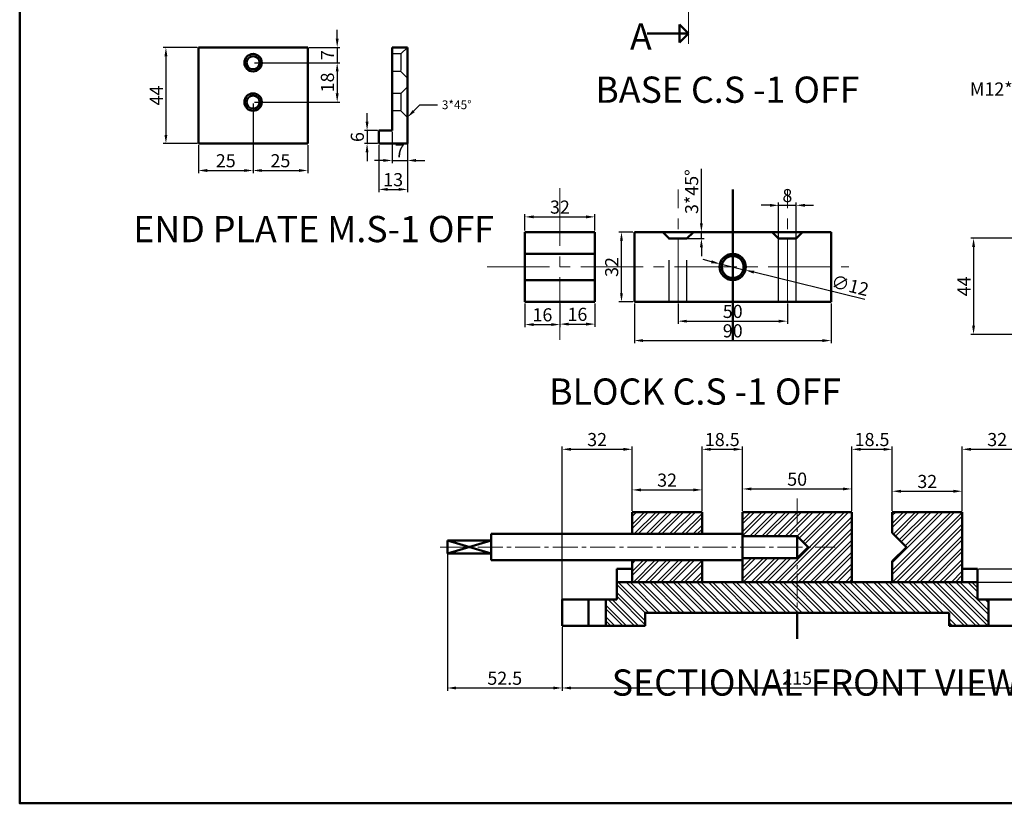
# Model space of a CAD drawing. Units: millimetres. Extents: x -1209 to -333, y 66 to 707.
# Tile 1 of 4: x -1209 to -759, y 66 to 424. Entities that reach past the tile are written whole.
import ezdxf
from ezdxf import colors
from ezdxf.entities.mleader import LeaderData, LeaderLine
from ezdxf.math import Vec2, Vec3

# ---------------------------------------------------------------- set-up
doc = ezdxf.new("R2010")
doc.units = ezdxf.units.MM
doc.header["$LTSCALE"] = 1.5
doc.linetypes.add('CENTER2', pattern=[28.575, 19.05, -3.175, 3.175, -3.175])
doc.linetypes.add('DASHED', pattern=[19.05, 12.7, -6.35])
for name, color, linetype, lineweight in [('M-CNTR', 1, 'CENTER2', 18), ('M-DIMS', 2, 'Continuous', 25), ('M-HATC', 8, 'Continuous', 18), ('M-HIDN', 4, 'DASHED', 25), ('M-OUTL', 7, 'Continuous', 50), ('M-TEXT', 3, 'Continuous', 25), ('M-TTLB', 7, 'Continuous', 50)]:
    doc.layers.add(name, color=color, linetype=linetype, lineweight=lineweight)
doc.styles.get("Standard").update_dxf_attribs({"font": 'arial.ttf'})
doc.dimstyles.new('ISO-25', dxfattribs={"dimtxt": 6, "dimasz": 4, "dimexe": 1.25, "dimexo": 0.625, "dimtad": 1, "dimdec": 0, "dimtxsty": 'Standard', "dimcen": 2.5, "dimadec": 0, "dimazin": 0, "dimtfac": 1, "dimtdec": 0, "dimtmove": 0, "dimatfit": 3, "dimfxl": 1, "dimarcsym": 0})

# ---------------------------------------------------------------- blocks, each defined once
blk = doc.blocks.new('*D29')
at = {"layer": 'Defpoints', "color": 0, "transparency": 16777216}
for p in [(-946, 334.25), (-978, 327.33), (-946, 327.33)]:
    blk.add_point(p, dxfattribs=at)
at = {"layer": 'M-DIMS', "color": 0, "lineweight": -2, "transparency": 16777216}
for p, q in [((-978, 327.95), (-978, 335.5)), ((-974, 334.25), (-950, 334.25)), ((-946, 327.95), (-946, 335.5))]:
    blk.add_line(p, q, dxfattribs=at)
at = {"layer": 'M-DIMS', "color": 0, "transparency": 16777216}
for points in [[(-974, 334.92), (-974, 333.58), (-978, 334.25)], [(-950, 334.92), (-950, 333.58), (-946, 334.25)]]:
    blk.add_solid(points, dxfattribs=at)
at = {"layer": 'M-DIMS', "color": 0, "transparency": 16777216, "insert": (-962, 337.94), "char_height": 6, "attachment_point": 5}
blk.add_mtext('32', dxfattribs=at)
blk = doc.blocks.new('*D30')
at = {"layer": 'Defpoints', "color": 0, "transparency": 16777216}
for p in [(-978, 295.33), (-962, 295.33), (-962, 284.99)]:
    blk.add_point(p, dxfattribs=at)
at = {"layer": 'M-DIMS', "color": 0, "lineweight": -2, "transparency": 16777216}
for p, q in [((-978, 294.7), (-978, 283.74)), ((-962, 294.7), (-962, 283.74)), ((-974, 284.99), (-966, 284.99))]:
    blk.add_line(p, q, dxfattribs=at)
at = {"layer": 'M-DIMS', "color": 0, "transparency": 16777216}
for points in [[(-974, 285.66), (-974, 284.32), (-978, 284.99)], [(-966, 285.66), (-966, 284.32), (-962, 284.99)]]:
    blk.add_solid(points, dxfattribs=at)
at = {"layer": 'M-DIMS', "color": 0, "transparency": 16777216, "insert": (-970, 288.68), "char_height": 6, "attachment_point": 5}
blk.add_mtext('16', dxfattribs=at)
blk = doc.blocks.new('*D31')
at = {"layer": 'Defpoints', "color": 0, "transparency": 16777216}
for p in [(-962, 295.33), (-946, 295.33), (-946, 285.2)]:
    blk.add_point(p, dxfattribs=at)
at = {"layer": 'M-DIMS', "color": 0, "lineweight": -2, "transparency": 16777216}
for p, q in [((-962, 294.7), (-962, 283.95)), ((-946, 294.7), (-946, 283.95)), ((-958, 285.2), (-950, 285.2))]:
    blk.add_line(p, q, dxfattribs=at)
at = {"layer": 'M-DIMS', "color": 0, "transparency": 16777216}
for points in [[(-958, 285.87), (-958, 284.53), (-962, 285.2)], [(-950, 285.87), (-950, 284.53), (-946, 285.2)]]:
    blk.add_solid(points, dxfattribs=at)
at = {"layer": 'M-DIMS', "color": 0, "transparency": 16777216, "insert": (-954, 288.89), "char_height": 6, "attachment_point": 5}
blk.add_mtext('16', dxfattribs=at)
blk = doc.blocks.new('*D32')
at = {"layer": 'Defpoints', "color": 0, "transparency": 16777216}
for p in [(-927.96, 295.33), (-837.96, 295.33), (-837.96, 277.67)]:
    blk.add_point(p, dxfattribs=at)
at = {"layer": 'M-DIMS', "color": 0, "lineweight": -2, "transparency": 16777216}
for p, q in [((-927.96, 294.7), (-927.96, 276.42)), ((-837.96, 294.7), (-837.96, 276.42)), ((-923.96, 277.67), (-841.96, 277.67))]:
    blk.add_line(p, q, dxfattribs=at)
at = {"layer": 'M-DIMS', "color": 0, "transparency": 16777216}
for points in [[(-923.96, 278.33), (-923.96, 277), (-927.96, 277.67)], [(-841.96, 278.33), (-841.96, 277), (-837.96, 277.67)]]:
    blk.add_solid(points, dxfattribs=at)
at = {"layer": 'M-DIMS', "color": 0, "transparency": 16777216, "insert": (-882.96, 281.35), "char_height": 6, "attachment_point": 5}
blk.add_mtext('90', dxfattribs=at)
blk = doc.blocks.new('*D33')
at = {"layer": 'Defpoints', "color": 0, "transparency": 16777216}
for p in [(-933.85, 327.33), (-927.96, 327.33), (-927.96, 295.33)]:
    blk.add_point(p, dxfattribs=at)
at = {"layer": 'M-DIMS', "color": 0, "lineweight": -2, "transparency": 16777216}
for p, q in [((-928.58, 327.33), (-935.1, 327.33)), ((-933.85, 299.33), (-933.85, 323.33)), ((-928.58, 295.33), (-935.1, 295.33))]:
    blk.add_line(p, q, dxfattribs=at)
at = {"layer": 'M-DIMS', "color": 0, "transparency": 16777216}
for points in [[(-934.51, 323.33), (-933.18, 323.33), (-933.85, 327.33)], [(-934.51, 299.33), (-933.18, 299.33), (-933.85, 295.33)]]:
    blk.add_solid(points, dxfattribs=at)
at = {"layer": 'M-DIMS', "color": 0, "transparency": 16777216, "insert": (-937.54, 311.33), "char_height": 6, "attachment_point": 5, "rotation": 90}
blk.add_mtext('32', dxfattribs=at)
blk = doc.blocks.new('*D34')
at = {"layer": 'Defpoints', "color": 0, "transparency": 16777216}
for p in [(-903.96, 327.33), (-903.96, 324.33), (-897.29, 327.33)]:
    blk.add_point(p, dxfattribs=at)
at = {"layer": 'M-DIMS', "color": 0, "lineweight": -2, "transparency": 16777216}
for p, q in [((-897.29, 331.33), (-897.29, 356.27)), ((-903.33, 327.33), (-896.04, 327.33)), ((-903.33, 324.33), (-896.04, 324.33)), ((-897.29, 324.33), (-897.29, 327.33)), ((-897.29, 320.33), (-897.29, 316.33))]:
    blk.add_line(p, q, dxfattribs=at)
at = {"layer": 'M-DIMS', "color": 0, "transparency": 16777216}
for points in [[(-897.95, 331.33), (-896.62, 331.33), (-897.29, 327.33)], [(-897.95, 320.33), (-896.62, 320.33), (-897.29, 324.33)]]:
    blk.add_solid(points, dxfattribs=at)
at = {"layer": 'M-DIMS', "color": 0, "transparency": 16777216, "insert": (-900.98, 345.8), "char_height": 6, "attachment_point": 5, "rotation": 90}
blk.add_mtext('3*45%%D', dxfattribs=at)
blk = doc.blocks.new('*D35')
at = {"layer": 'Defpoints', "color": 0, "transparency": 16777216}
for p in [(-907.96, 295.33), (-857.96, 295.33), (-857.96, 286.54)]:
    blk.add_point(p, dxfattribs=at)
at = {"layer": 'M-DIMS', "color": 0, "lineweight": -2, "transparency": 16777216}
for p, q in [((-907.96, 294.7), (-907.96, 285.29)), ((-857.96, 294.7), (-857.96, 285.29)), ((-903.96, 286.54), (-861.96, 286.54))]:
    blk.add_line(p, q, dxfattribs=at)
at = {"layer": 'M-DIMS', "color": 0, "transparency": 16777216}
for points in [[(-903.96, 287.2), (-903.96, 285.87), (-907.96, 286.54)], [(-861.96, 287.2), (-861.96, 285.87), (-857.96, 286.54)]]:
    blk.add_solid(points, dxfattribs=at)
at = {"layer": 'M-DIMS', "color": 0, "transparency": 16777216, "insert": (-882.96, 290.23), "char_height": 6, "attachment_point": 5}
blk.add_mtext('50', dxfattribs=at)
blk = doc.blocks.new('*D36')
at = {"layer": 'Defpoints', "color": 0, "transparency": 16777216}
for p in [(-888.78, 312.76), (-877.13, 309.89)]:
    blk.add_point(p, dxfattribs=at)
at = {"layer": 'M-DIMS', "color": 0, "lineweight": -2, "transparency": 16777216}
for p, q in [((-892.67, 313.72), (-896.55, 314.68)), ((-888.78, 312.76), (-877.13, 309.89)), ((-822.47, 296.42), (-873.25, 308.93))]:
    blk.add_line(p, q, dxfattribs=at)
at = {"layer": 'M-DIMS', "color": 0, "transparency": 16777216}
for points in [[(-892.51, 314.37), (-892.83, 313.07), (-888.78, 312.76)], [(-873.09, 309.58), (-873.41, 308.29), (-877.13, 309.89)]]:
    blk.add_solid(points, dxfattribs=at)
at = {"layer": 'M-DIMS', "color": 0, "transparency": 16777216, "insert": (-829.47, 302.12), "char_height": 6, "attachment_point": 5, "rotation": 346.1592}
blk.add_mtext('∅12', dxfattribs=at)
blk = doc.blocks.new('*D37')
at = {"layer": 'Defpoints', "color": 0, "transparency": 16777216}
for p in [(-853.96, 339.53), (-861.96, 311.33), (-853.96, 311.33)]:
    blk.add_point(p, dxfattribs=at)
at = {"layer": 'M-DIMS', "color": 0, "lineweight": -2, "transparency": 16777216}
for p, q in [((-865.96, 339.53), (-869.96, 339.53)), ((-861.96, 311.95), (-861.96, 340.78)), ((-861.96, 339.53), (-853.96, 339.53)), ((-853.96, 311.95), (-853.96, 340.78)), ((-849.96, 339.53), (-845.96, 339.53))]:
    blk.add_line(p, q, dxfattribs=at)
at = {"layer": 'M-DIMS', "color": 0, "transparency": 16777216}
for points in [[(-865.96, 340.2), (-865.96, 338.87), (-861.96, 339.53)], [(-849.96, 340.2), (-849.96, 338.87), (-853.96, 339.53)]]:
    blk.add_solid(points, dxfattribs=at)
at = {"layer": 'M-DIMS', "color": 0, "transparency": 16777216, "insert": (-857.96, 343.22), "char_height": 6, "attachment_point": 5}
blk.add_mtext('8', dxfattribs=at)
blk = doc.blocks.new('*D40')
at = {"layer": 'Defpoints', "color": 0, "transparency": 16777216}
for p in [(-752.7, 324.49), (-772.81, 280.49), (-752.7, 280.49)]:
    blk.add_point(p, dxfattribs=at)
at = {"layer": 'M-DIMS', "color": 0, "lineweight": -2, "transparency": 16777216}
for p, q in [((-753.33, 324.49), (-774.06, 324.49)), ((-772.81, 320.49), (-772.81, 284.49)), ((-753.33, 280.49), (-774.06, 280.49))]:
    blk.add_line(p, q, dxfattribs=at)
at = {"layer": 'M-DIMS', "color": 0, "transparency": 16777216}
for points in [[(-773.47, 320.49), (-772.14, 320.49), (-772.81, 324.49)], [(-773.47, 284.49), (-772.14, 284.49), (-772.81, 280.49)]]:
    blk.add_solid(points, dxfattribs=at)
at = {"layer": 'M-DIMS', "color": 0, "transparency": 16777216, "insert": (-776.43, 302.49), "char_height": 6, "attachment_point": 5, "rotation": 90}
blk.add_mtext('44', dxfattribs=at)
blk = doc.blocks.new('*D63')
at = {"layer": 'Defpoints', "color": 0, "ltscale": 0.4, "transparency": 16777216}
for p in [(-1127.34, 411.75), (-1142.21, 367.75), (-1127.34, 367.75)]:
    blk.add_point(p, dxfattribs=at)
at = {"layer": 'M-DIMS', "color": 0, "lineweight": -2, "ltscale": 0.4, "transparency": 16777216}
for p, q in [((-1127.97, 411.75), (-1143.46, 411.75)), ((-1142.21, 407.75), (-1142.21, 371.75)), ((-1127.97, 367.75), (-1143.46, 367.75))]:
    blk.add_line(p, q, dxfattribs=at)
at = {"layer": 'M-DIMS', "color": 0, "ltscale": 0.4, "transparency": 16777216}
for points in [[(-1142.87, 407.75), (-1141.54, 407.75), (-1142.21, 411.75)], [(-1142.87, 371.75), (-1141.54, 371.75), (-1142.21, 367.75)]]:
    blk.add_solid(points, dxfattribs=at)
at = {"layer": 'M-DIMS', "color": 0, "ltscale": 0.4, "transparency": 16777216, "insert": (-1145.83, 389.75), "char_height": 6, "attachment_point": 5, "rotation": 90}
blk.add_mtext('44', dxfattribs=at)
blk = doc.blocks.new('*D64')
at = {"layer": 'Defpoints', "color": 0, "ltscale": 0.4, "transparency": 16777216}
for p in [(-1077.34, 411.75), (-1102.34, 404.75), (-1063.87, 404.75)]:
    blk.add_point(p, dxfattribs=at)
at = {"layer": 'M-DIMS', "color": 0, "lineweight": -2, "ltscale": 0.4, "transparency": 16777216}
for p, q in [((-1063.87, 415.75), (-1063.87, 419.75)), ((-1076.72, 411.75), (-1062.62, 411.75)), ((-1063.87, 411.75), (-1063.87, 404.75)), ((-1101.72, 404.75), (-1062.62, 404.75)), ((-1063.87, 400.75), (-1063.87, 396.75))]:
    blk.add_line(p, q, dxfattribs=at)
at = {"layer": 'M-DIMS', "color": 0, "ltscale": 0.4, "transparency": 16777216}
for points in [[(-1064.54, 415.75), (-1063.21, 415.75), (-1063.87, 411.75)], [(-1064.54, 400.75), (-1063.21, 400.75), (-1063.87, 404.75)]]:
    blk.add_solid(points, dxfattribs=at)
at = {"layer": 'M-DIMS', "color": 0, "ltscale": 0.4, "transparency": 16777216, "insert": (-1067.5, 408.25), "char_height": 6, "attachment_point": 5, "rotation": 90}
blk.add_mtext('7', dxfattribs=at)
blk = doc.blocks.new('*D65')
at = {"layer": 'Defpoints', "color": 0, "ltscale": 0.4, "transparency": 16777216}
for p in [(-1077.34, 404.75), (-1102.34, 386.75), (-1063.87, 386.75)]:
    blk.add_point(p, dxfattribs=at)
at = {"layer": 'M-DIMS', "color": 0, "lineweight": -2, "ltscale": 0.4, "transparency": 16777216}
for p, q in [((-1076.72, 404.75), (-1062.62, 404.75)), ((-1063.87, 400.75), (-1063.87, 390.75)), ((-1101.72, 386.75), (-1062.62, 386.75))]:
    blk.add_line(p, q, dxfattribs=at)
at = {"layer": 'M-DIMS', "color": 0, "ltscale": 0.4, "transparency": 16777216}
for points in [[(-1064.54, 400.75), (-1063.21, 400.75), (-1063.87, 404.75)], [(-1064.54, 390.75), (-1063.21, 390.75), (-1063.87, 386.75)]]:
    blk.add_solid(points, dxfattribs=at)
at = {"layer": 'M-DIMS', "color": 0, "ltscale": 0.4, "transparency": 16777216, "insert": (-1067.56, 395.75), "char_height": 6, "attachment_point": 5, "rotation": 90}
blk.add_mtext('18', dxfattribs=at)
blk = doc.blocks.new('*D66')
at = {"layer": 'Defpoints', "color": 0, "ltscale": 0.4, "transparency": 16777216}
for p in [(-1102.34, 386.75), (-1127.34, 367.75), (-1102.34, 355.46)]:
    blk.add_point(p, dxfattribs=at)
at = {"layer": 'M-DIMS', "color": 0, "lineweight": -2, "ltscale": 0.4, "transparency": 16777216}
for p, q in [((-1102.34, 386.12), (-1102.34, 354.21)), ((-1127.34, 367.12), (-1127.34, 354.21)), ((-1123.34, 355.46), (-1106.34, 355.46))]:
    blk.add_line(p, q, dxfattribs=at)
at = {"layer": 'M-DIMS', "color": 0, "ltscale": 0.4, "transparency": 16777216}
for points in [[(-1123.34, 356.13), (-1123.34, 354.79), (-1127.34, 355.46)], [(-1106.34, 356.13), (-1106.34, 354.79), (-1102.34, 355.46)]]:
    blk.add_solid(points, dxfattribs=at)
at = {"layer": 'M-DIMS', "color": 0, "ltscale": 0.4, "transparency": 16777216, "insert": (-1114.84, 359.15), "char_height": 6, "attachment_point": 5}
blk.add_mtext('25', dxfattribs=at)
blk = doc.blocks.new('*D67')
at = {"layer": 'Defpoints', "color": 0, "ltscale": 0.4, "transparency": 16777216}
for p in [(-1102.34, 386.75), (-1077.34, 367.75), (-1077.34, 355.46)]:
    blk.add_point(p, dxfattribs=at)
at = {"layer": 'M-DIMS', "color": 0, "lineweight": -2, "ltscale": 0.4, "transparency": 16777216}
for p, q in [((-1102.34, 386.12), (-1102.34, 354.21)), ((-1077.34, 367.12), (-1077.34, 354.21)), ((-1098.34, 355.46), (-1081.34, 355.46))]:
    blk.add_line(p, q, dxfattribs=at)
at = {"layer": 'M-DIMS', "color": 0, "ltscale": 0.4, "transparency": 16777216}
for points in [[(-1098.34, 356.13), (-1098.34, 354.79), (-1102.34, 355.46)], [(-1081.34, 356.13), (-1081.34, 354.79), (-1077.34, 355.46)]]:
    blk.add_solid(points, dxfattribs=at)
at = {"layer": 'M-DIMS', "color": 0, "ltscale": 0.4, "transparency": 16777216, "insert": (-1089.84, 359.15), "char_height": 6, "attachment_point": 5}
blk.add_mtext('25', dxfattribs=at)
blk = doc.blocks.new('*D68')
at = {"layer": 'Defpoints', "color": 0, "ltscale": 0.4, "transparency": 16777216}
for p in [(-1044.77, 367.75), (-1031.77, 367.75), (-1031.77, 346.81)]:
    blk.add_point(p, dxfattribs=at)
at = {"layer": 'M-DIMS', "color": 0, "lineweight": -2, "ltscale": 0.4, "transparency": 16777216}
for p, q in [((-1044.77, 367.12), (-1044.77, 345.56)), ((-1031.77, 367.12), (-1031.77, 345.56)), ((-1040.77, 346.81), (-1035.77, 346.81))]:
    blk.add_line(p, q, dxfattribs=at)
at = {"layer": 'M-DIMS', "color": 0, "ltscale": 0.4, "transparency": 16777216}
for points in [[(-1040.77, 347.48), (-1040.77, 346.15), (-1044.77, 346.81)], [(-1035.77, 347.48), (-1035.77, 346.15), (-1031.77, 346.81)]]:
    blk.add_solid(points, dxfattribs=at)
at = {"layer": 'M-DIMS', "color": 0, "ltscale": 0.4, "transparency": 16777216, "insert": (-1038.27, 350.5), "char_height": 6, "attachment_point": 5}
blk.add_mtext('13', dxfattribs=at)
blk = doc.blocks.new('*D69')
at = {"layer": 'Defpoints', "color": 0, "ltscale": 0.4, "transparency": 16777216}
for p in [(-1038.77, 373.75), (-1031.77, 373.75), (-1031.77, 360.05)]:
    blk.add_point(p, dxfattribs=at)
at = {"layer": 'M-DIMS', "color": 0, "lineweight": -2, "ltscale": 0.4, "transparency": 16777216}
for p, q in [((-1038.77, 373.12), (-1038.77, 358.8)), ((-1031.77, 373.12), (-1031.77, 358.8)), ((-1042.77, 360.05), (-1046.77, 360.05)), ((-1038.77, 360.05), (-1031.77, 360.05)), ((-1027.77, 360.05), (-1023.77, 360.05))]:
    blk.add_line(p, q, dxfattribs=at)
at = {"layer": 'M-DIMS', "color": 0, "ltscale": 0.4, "transparency": 16777216}
for points in [[(-1042.77, 360.72), (-1042.77, 359.39), (-1038.77, 360.05)], [(-1027.77, 360.72), (-1027.77, 359.39), (-1031.77, 360.05)]]:
    blk.add_solid(points, dxfattribs=at)
at = {"layer": 'M-DIMS', "color": 0, "ltscale": 0.4, "transparency": 16777216, "insert": (-1035.27, 363.68), "char_height": 6, "attachment_point": 5}
blk.add_mtext('7', dxfattribs=at)
blk = doc.blocks.new('*D70')
at = {"layer": 'Defpoints', "color": 0, "ltscale": 0.4, "transparency": 16777216}
for p in [(-1044.77, 373.75), (-1050.2, 367.75), (-1044.77, 367.75)]:
    blk.add_point(p, dxfattribs=at)
at = {"layer": 'M-DIMS', "color": 0, "lineweight": -2, "ltscale": 0.4, "transparency": 16777216}
for p, q in [((-1050.2, 377.75), (-1050.2, 381.75)), ((-1045.4, 373.75), (-1051.45, 373.75)), ((-1050.2, 373.75), (-1050.2, 367.75)), ((-1045.4, 367.75), (-1051.45, 367.75)), ((-1050.2, 363.75), (-1050.2, 359.75))]:
    blk.add_line(p, q, dxfattribs=at)
at = {"layer": 'M-DIMS', "color": 0, "ltscale": 0.4, "transparency": 16777216}
for points in [[(-1050.87, 377.75), (-1049.54, 377.75), (-1050.2, 373.75)], [(-1050.87, 363.75), (-1049.54, 363.75), (-1050.2, 367.75)]]:
    blk.add_solid(points, dxfattribs=at)
at = {"layer": 'M-DIMS', "color": 0, "ltscale": 0.4, "transparency": 16777216, "insert": (-1053.89, 370.75), "char_height": 6, "attachment_point": 5, "rotation": 90}
blk.add_mtext('6', dxfattribs=at)
blk = doc.blocks.new('*D72')
at = {"layer": 'Defpoints', "color": 0, "ltscale": 0.4, "transparency": 16777216}
for p in [(-896.99, 209.36), (-928.99, 199.2), (-896.99, 199.2)]:
    blk.add_point(p, dxfattribs=at)
at = {"layer": 'M-DIMS', "color": 0, "lineweight": -2, "ltscale": 0.4, "transparency": 16777216}
for p, q in [((-928.99, 199.83), (-928.99, 210.61)), ((-924.99, 209.36), (-900.99, 209.36)), ((-896.99, 199.83), (-896.99, 210.61))]:
    blk.add_line(p, q, dxfattribs=at)
at = {"layer": 'M-DIMS', "color": 0, "ltscale": 0.4, "transparency": 16777216}
for points in [[(-924.99, 210.03), (-924.99, 208.7), (-928.99, 209.36)], [(-900.99, 210.03), (-900.99, 208.7), (-896.99, 209.36)]]:
    blk.add_solid(points, dxfattribs=at)
at = {"layer": 'M-DIMS', "color": 0, "ltscale": 0.4, "transparency": 16777216, "insert": (-912.99, 213.05), "char_height": 6, "attachment_point": 5}
blk.add_mtext('32', dxfattribs=at)
blk = doc.blocks.new('*D73')
at = {"layer": 'Defpoints', "color": 0, "ltscale": 0.4, "transparency": 16777216}
for p in [(-828.49, 209.8), (-878.49, 199.2), (-828.49, 199.2)]:
    blk.add_point(p, dxfattribs=at)
at = {"layer": 'M-DIMS', "color": 0, "lineweight": -2, "ltscale": 0.4, "transparency": 16777216}
for p, q in [((-878.49, 199.83), (-878.49, 211.05)), ((-874.49, 209.8), (-832.49, 209.8)), ((-828.49, 199.83), (-828.49, 211.05))]:
    blk.add_line(p, q, dxfattribs=at)
at = {"layer": 'M-DIMS', "color": 0, "ltscale": 0.4, "transparency": 16777216}
for points in [[(-874.49, 210.47), (-874.49, 209.14), (-878.49, 209.8)], [(-832.49, 210.47), (-832.49, 209.14), (-828.49, 209.8)]]:
    blk.add_solid(points, dxfattribs=at)
at = {"layer": 'M-DIMS', "color": 0, "ltscale": 0.4, "transparency": 16777216, "insert": (-853.49, 213.49), "char_height": 6, "attachment_point": 5}
blk.add_mtext('50', dxfattribs=at)
blk = doc.blocks.new('*D74')
at = {"layer": 'Defpoints', "color": 0, "ltscale": 0.4, "transparency": 16777216}
for p in [(-777.99, 208.75), (-809.99, 199.2), (-777.99, 199.2)]:
    blk.add_point(p, dxfattribs=at)
at = {"layer": 'M-DIMS', "color": 0, "lineweight": -2, "ltscale": 0.4, "transparency": 16777216}
for p, q in [((-809.99, 199.83), (-809.99, 210)), ((-805.99, 208.75), (-781.99, 208.75)), ((-777.99, 199.83), (-777.99, 210))]:
    blk.add_line(p, q, dxfattribs=at)
at = {"layer": 'M-DIMS', "color": 0, "ltscale": 0.4, "transparency": 16777216}
for points in [[(-805.99, 209.42), (-805.99, 208.08), (-809.99, 208.75)], [(-781.99, 209.42), (-781.99, 208.08), (-777.99, 208.75)]]:
    blk.add_solid(points, dxfattribs=at)
at = {"layer": 'M-DIMS', "color": 0, "ltscale": 0.4, "transparency": 16777216, "insert": (-793.99, 212.44), "char_height": 6, "attachment_point": 5}
blk.add_mtext('32', dxfattribs=at)
blk = doc.blocks.new('*D75')
at = {"layer": 'Defpoints', "color": 0, "ltscale": 0.4, "transparency": 16777216}
for p in [(-770.99, 173.2), (-770.99, 167.2), (-735.83, 167.2)]:
    blk.add_point(p, dxfattribs=at)
at = {"layer": 'M-DIMS', "color": 0, "lineweight": -2, "ltscale": 0.4, "transparency": 16777216}
for p, q in [((-735.83, 177.2), (-735.83, 181.2)), ((-770.37, 173.2), (-734.58, 173.2)), ((-735.83, 173.2), (-735.83, 167.2)), ((-770.37, 167.2), (-734.58, 167.2)), ((-735.83, 163.2), (-735.83, 159.2))]:
    blk.add_line(p, q, dxfattribs=at)
at = {"layer": 'M-DIMS', "color": 0, "ltscale": 0.4, "transparency": 16777216}
for points in [[(-736.5, 177.2), (-735.16, 177.2), (-735.83, 173.2)], [(-736.5, 163.2), (-735.16, 163.2), (-735.83, 167.2)]]:
    blk.add_solid(points, dxfattribs=at)
at = {"layer": 'M-DIMS', "color": 0, "ltscale": 0.4, "transparency": 16777216, "insert": (-739.52, 170.2), "char_height": 6, "attachment_point": 5, "rotation": 90}
blk.add_mtext('6', dxfattribs=at)
blk = doc.blocks.new('*D79')
at = {"layer": 'Defpoints', "color": 0, "ltscale": 1.5, "transparency": 16777216}
for p in [(-928.99, 227.93), (-928.99, 199.2), (-960.99, 147.2)]:
    blk.add_point(p, dxfattribs=at)
at = {"layer": 'M-DIMS', "color": 0, "lineweight": -2, "ltscale": 1.5, "transparency": 16777216}
for p, q in [((-960.99, 147.83), (-960.99, 229.18)), ((-956.99, 227.93), (-932.99, 227.93)), ((-928.99, 199.83), (-928.99, 229.18))]:
    blk.add_line(p, q, dxfattribs=at)
at = {"layer": 'M-DIMS', "color": 0, "ltscale": 1.5, "transparency": 16777216}
for points in [[(-956.99, 228.6), (-956.99, 227.26), (-960.99, 227.93)], [(-932.99, 228.6), (-932.99, 227.26), (-928.99, 227.93)]]:
    blk.add_solid(points, dxfattribs=at)
at = {"layer": 'M-DIMS', "color": 0, "ltscale": 1.5, "transparency": 16777216, "insert": (-944.99, 231.62), "char_height": 6, "attachment_point": 5}
blk.add_mtext('32', dxfattribs=at)
blk = doc.blocks.new('*D80')
at = {"layer": 'Defpoints', "color": 0, "ltscale": 1.5, "transparency": 16777216}
for p in [(-878.49, 227.93), (-896.99, 199.2), (-878.49, 199.2)]:
    blk.add_point(p, dxfattribs=at)
at = {"layer": 'M-DIMS', "color": 0, "lineweight": -2, "ltscale": 1.5, "transparency": 16777216}
for p, q in [((-896.99, 199.83), (-896.99, 229.18)), ((-892.99, 227.93), (-882.49, 227.93)), ((-878.49, 199.83), (-878.49, 229.18))]:
    blk.add_line(p, q, dxfattribs=at)
at = {"layer": 'M-DIMS', "color": 0, "ltscale": 1.5, "transparency": 16777216}
for points in [[(-892.99, 228.6), (-892.99, 227.26), (-896.99, 227.93)], [(-882.49, 228.6), (-882.49, 227.26), (-878.49, 227.93)]]:
    blk.add_solid(points, dxfattribs=at)
at = {"layer": 'M-DIMS', "color": 0, "ltscale": 1.5, "transparency": 16777216, "insert": (-887.74, 231.62), "char_height": 6, "attachment_point": 5}
blk.add_mtext('18.5', dxfattribs=at)
blk = doc.blocks.new('*D81')
at = {"layer": 'Defpoints', "color": 0, "ltscale": 1.5, "transparency": 16777216}
for p in [(-809.99, 227.93), (-828.49, 199.2), (-809.99, 199.2)]:
    blk.add_point(p, dxfattribs=at)
at = {"layer": 'M-DIMS', "color": 0, "lineweight": -2, "ltscale": 1.5, "transparency": 16777216}
for p, q in [((-828.49, 199.83), (-828.49, 229.18)), ((-824.49, 227.93), (-813.99, 227.93)), ((-809.99, 199.83), (-809.99, 229.18))]:
    blk.add_line(p, q, dxfattribs=at)
at = {"layer": 'M-DIMS', "color": 0, "ltscale": 1.5, "transparency": 16777216}
for points in [[(-824.49, 228.6), (-824.49, 227.26), (-828.49, 227.93)], [(-813.99, 228.6), (-813.99, 227.26), (-809.99, 227.93)]]:
    blk.add_solid(points, dxfattribs=at)
at = {"layer": 'M-DIMS', "color": 0, "ltscale": 1.5, "transparency": 16777216, "insert": (-819.24, 231.62), "char_height": 6, "attachment_point": 5}
blk.add_mtext('18.5', dxfattribs=at)
blk = doc.blocks.new('*D82')
at = {"layer": 'Defpoints', "color": 0, "ltscale": 1.5, "transparency": 16777216}
for p in [(-745.99, 227.93), (-777.99, 199.2), (-745.99, 147.2)]:
    blk.add_point(p, dxfattribs=at)
at = {"layer": 'M-DIMS', "color": 0, "lineweight": -2, "ltscale": 1.5, "transparency": 16777216}
for p, q in [((-777.99, 199.83), (-777.99, 229.18)), ((-773.99, 227.93), (-749.99, 227.93)), ((-745.99, 147.83), (-745.99, 229.18))]:
    blk.add_line(p, q, dxfattribs=at)
at = {"layer": 'M-DIMS', "color": 0, "ltscale": 1.5, "transparency": 16777216}
for points in [[(-773.99, 228.6), (-773.99, 227.26), (-777.99, 227.93)], [(-749.99, 228.6), (-749.99, 227.26), (-745.99, 227.93)]]:
    blk.add_solid(points, dxfattribs=at)
at = {"layer": 'M-DIMS', "color": 0, "ltscale": 1.5, "transparency": 16777216, "insert": (-761.99, 231.62), "char_height": 6, "attachment_point": 5}
blk.add_mtext('32', dxfattribs=at)
blk = doc.blocks.new('*D83')
at = {"layer": 'Defpoints', "color": 0, "ltscale": 1.5, "transparency": 16777216}
for p in [(-960.99, 147.2), (-745.99, 147.2), (-745.99, 118.76)]:
    blk.add_point(p, dxfattribs=at)
at = {"layer": 'M-DIMS', "color": 0, "lineweight": -2, "ltscale": 1.5, "transparency": 16777216}
for p, q in [((-960.99, 146.58), (-960.99, 117.51)), ((-745.99, 146.58), (-745.99, 117.51)), ((-956.99, 118.76), (-749.99, 118.76))]:
    blk.add_line(p, q, dxfattribs=at)
at = {"layer": 'M-DIMS', "color": 0, "ltscale": 1.5, "transparency": 16777216}
for points in [[(-956.99, 119.42), (-956.99, 118.09), (-960.99, 118.76)], [(-749.99, 119.42), (-749.99, 118.09), (-745.99, 118.76)]]:
    blk.add_solid(points, dxfattribs=at)
at = {"layer": 'M-DIMS', "color": 0, "ltscale": 1.5, "transparency": 16777216, "insert": (-853.49, 122.44), "char_height": 6, "attachment_point": 5}
blk.add_mtext('215', dxfattribs=at)
blk = doc.blocks.new('*D84')
at = {"layer": 'Defpoints', "color": 0, "ltscale": 1.5, "transparency": 16777216}
for p in [(-1013.49, 186.2), (-960.99, 147.2), (-960.99, 118.76)]:
    blk.add_point(p, dxfattribs=at)
at = {"layer": 'M-DIMS', "color": 0, "lineweight": -2, "ltscale": 1.5, "transparency": 16777216}
for p, q in [((-1013.49, 185.58), (-1013.49, 117.51)), ((-960.99, 146.58), (-960.99, 117.51)), ((-1009.49, 118.76), (-964.99, 118.76))]:
    blk.add_line(p, q, dxfattribs=at)
at = {"layer": 'M-DIMS', "color": 0, "ltscale": 1.5, "transparency": 16777216}
for points in [[(-1009.49, 119.42), (-1009.49, 118.09), (-1013.49, 118.76)], [(-964.99, 119.42), (-964.99, 118.09), (-960.99, 118.76)]]:
    blk.add_solid(points, dxfattribs=at)
at = {"layer": 'M-DIMS', "color": 0, "ltscale": 1.5, "transparency": 16777216, "insert": (-987.24, 122.44), "char_height": 6, "attachment_point": 5}
blk.add_mtext('52.5', dxfattribs=at)

msp = doc.modelspace()

# ---------------------------------------------------------------- hatches: boundary and pattern name
at = {"layer": 'M-HATC', "ltscale": 0.4}
h = msp.add_hatch(dxfattribs=at)
h.set_pattern_fill('ANSI32', color=256, scale=0.4)
h.set_pattern_definition([(45, (-1404.2333, -437.927), (-2.694077, 2.694077), []), (45, (-1402.4373, -437.927), (-2.694077, 2.694077), [])])
h.paths.add_polyline_path([(-896.99, 199.2), (-928.99, 199.2), (-928.99, 189.2), (-896.99, 189.2)])
h.paths.add_polyline_path([(-853.49, 199.2), (-878.49, 199.2), (-878.49, 188.2), (-853.49, 188.2)])
h.paths.add_polyline_path([(-828.49, 199.2), (-853.49, 199.2), (-853.49, 188.2), (-848.49, 183.2), (-853.49, 178.2), (-853.49, 167.2), (-828.49, 167.2)])
h.paths.add_polyline_path([(-853.49, 178.2), (-878.49, 178.2), (-878.49, 167.2), (-853.49, 167.2)])
h.paths.add_polyline_path([(-896.99, 177.2), (-928.99, 177.2), (-928.99, 167.2), (-896.99, 167.2)])
h.paths.add_polyline_path([(-777.99, 199.2), (-809.99, 199.2), (-809.99, 189.7), (-803.49, 183.2), (-809.99, 176.7), (-809.99, 167.2), (-777.99, 167.2), (-777.99, 173.2)])
h = msp.add_hatch(dxfattribs=at)
h.set_pattern_fill('ANSI32', color=256, scale=0.4, angle=90)
h.set_pattern_definition([(135, (-1404.2333, -437.927), (-2.694077, -2.694077), []), (135, (-1404.2333, -436.131), (-2.694077, -2.694077), [])])
h.paths.add_polyline_path([(-853.49, 167.2), (-865.99, 167.2), (-935.99, 167.2), (-935.99, 159.2), (-940.99, 159.2), (-940.99, 147.2), (-922.99, 147.2), (-922.99, 153.2), (-853.49, 153.2)])
h.paths.add_polyline_path([(-770.99, 167.2), (-853.49, 167.2), (-853.49, 153.2), (-783.99, 153.2), (-783.99, 147.2), (-765.99, 147.2), (-765.99, 159.2), (-770.99, 159.2)])

# ---------------------------------------------------------------- linework, layer by layer
at = {"layer": 'M-CNTR'}
for p, q in [((-903.18, 413.37), (-903.18, 617.86)), ((-962, 278.08), (-962, 347.35)), ((-907.96, 295.33), (-907.96, 346.72)), ((-857.96, 295.33), (-857.96, 346.72)), ((-995.35, 311.33), (-829.86, 311.33))]:
    msp.add_line(p, q, dxfattribs=at)
at = {"layer": 'M-CNTR', "ltscale": 0.4}
for p, q in [((-853.49, 205.43), (-853.49, 153.2)), ((-1016.74, 183.2), (-836.17, 183.2))]:
    msp.add_line(p, q, dxfattribs=at)
at = {"layer": 'M-HIDN', "ltscale": 0.4}
for p, q in [((-1034.77, 408.75), (-1031.77, 411.75)), ((-1034.77, 408.75), (-1038.77, 408.75)), ((-1034.77, 408.75), (-1034.77, 400.75)), ((-1034.77, 400.75), (-1038.77, 400.75)), ((-1034.77, 400.75), (-1031.77, 397.75)), ((-1034.77, 390.75), (-1031.77, 393.75)), ((-1034.77, 390.75), (-1038.77, 390.75)), ((-1034.77, 390.75), (-1034.77, 382.75)), ((-1034.77, 382.75), (-1038.77, 382.75)), ((-1034.77, 382.75), (-1031.77, 379.75))]:
    msp.add_line(p, q, dxfattribs=at)
at = {"layer": 'M-HIDN'}
for p, q in [((-911.96, 295.33), (-911.96, 324.33)), ((-903.96, 295.33), (-903.96, 324.33)), ((-861.96, 295.33), (-861.96, 324.33)), ((-853.96, 295.33), (-853.96, 324.33))]:
    msp.add_line(p, q, dxfattribs=at)
at = {"layer": 'M-OUTL', "ltscale": 0.4}
for p, q in [((-903.18, 418.12), (-907.36, 422.3)), ((-907.36, 422.3), (-907.36, 413.94)), ((-903.18, 418.12), (-922.06, 418.12)), ((-903.18, 418.12), (-907.36, 413.94)), ((-1034.77, 411.75), (-1038.77, 411.75)), ((-1038.77, 411.75), (-1038.77, 373.75)), ((-1031.77, 411.75), (-1034.77, 411.75)), ((-1031.77, 367.75), (-1031.77, 411.75)), ((-1038.77, 373.75), (-1044.77, 373.75)), ((-1044.77, 373.75), (-1044.77, 367.75)), ((-1044.77, 367.75), (-1031.77, 367.75)), ((-928.99, 199.2), (-896.99, 199.2)), ((-928.99, 189.2), (-928.99, 199.2)), ((-896.99, 199.2), (-896.99, 189.2)), ((-828.49, 199.2), (-878.49, 199.2)), ((-878.49, 199.2), (-878.49, 167.2)), ((-828.49, 167.2), (-828.49, 199.2)), ((-777.99, 199.2), (-809.99, 199.2)), ((-809.99, 199.2), (-809.99, 189.7)), ((-777.99, 167.2), (-777.99, 199.2)), ((-809.99, 189.7), (-803.49, 183.2)), ((-853.49, 188.2), (-848.49, 183.2)), ((-853.49, 178.2), (-848.49, 183.2)), ((-809.99, 176.7), (-803.49, 183.2)), ((-928.99, 167.2), (-928.99, 177.2)), ((-896.99, 177.2), (-896.99, 167.2)), ((-809.99, 176.7), (-809.99, 167.2)), ((-935.99, 159.2), (-935.99, 173.2)), ((-935.99, 173.2), (-928.99, 173.2)), ((-928.99, 173.2), (-928.99, 167.2)), ((-770.99, 173.2), (-777.99, 173.2)), ((-777.99, 173.2), (-777.99, 167.2)), ((-770.99, 159.2), (-770.99, 173.2)), ((-935.99, 167.2), (-853.49, 167.2)), ((-853.49, 167.2), (-865.99, 167.2)), ((-770.99, 167.2), (-853.49, 167.2)), ((-853.49, 167.2), (-840.99, 167.2)), ((-853.49, 167.2), (-828.49, 167.2)), ((-960.99, 147.2), (-960.99, 159.2)), ((-960.99, 159.2), (-935.99, 159.2)), ((-948.99, 147.2), (-948.99, 159.2)), ((-940.99, 147.2), (-940.99, 159.2)), ((-745.99, 159.2), (-770.99, 159.2)), ((-765.99, 147.2), (-765.99, 159.2)), ((-853.49, 153.2), (-922.99, 153.2)), ((-922.99, 147.2), (-922.99, 153.2)), ((-853.49, 153.2), (-783.99, 153.2)), ((-853.49, 153.2), (-853.49, 141.26)), ((-783.99, 147.2), (-783.99, 153.2)), ((-922.99, 147.2), (-960.99, 147.2)), ((-783.99, 147.2), (-745.99, 147.2))]:
    msp.add_line(p, q, dxfattribs=at)
at = {"layer": 'M-OUTL'}
for p, q in [((-1077.34, 411.75), (-1127.34, 411.75)), ((-1127.34, 411.75), (-1127.34, 367.75)), ((-1077.34, 395.75), (-1077.34, 411.75)), ((-1077.34, 367.75), (-1077.34, 395.75)), ((-1127.34, 367.75), (-1102.34, 367.75)), ((-1102.34, 367.75), (-1077.34, 367.75)), ((-882.96, 277.67), (-882.96, 346.72)), ((-978, 311.33), (-978, 327.33)), ((-978, 327.33), (-946, 327.33)), ((-946, 327.33), (-946, 295.33)), ((-927.96, 311.33), (-927.96, 327.33)), ((-927.96, 327.33), (-837.96, 327.33)), ((-911.96, 324.33), (-914.92, 327.33)), ((-911.96, 324.33), (-903.96, 324.33)), ((-903.96, 324.33), (-900.93, 327.33)), ((-861.96, 324.33), (-864.97, 327.33)), ((-861.96, 324.33), (-853.96, 324.33)), ((-853.96, 324.33), (-851, 327.33)), ((-837.96, 327.33), (-837.96, 295.33)), ((-978, 317.33), (-946, 317.33)), ((-978, 295.33), (-978, 311.33)), ((-927.96, 295.33), (-927.96, 311.33)), ((-978, 305.33), (-946, 305.33)), ((-946, 295.33), (-978, 295.33)), ((-837.96, 295.33), (-927.96, 295.33)), ((-993.49, 178.2), (-993.49, 189.2)), ((-993.49, 189.2), (-935.49, 189.2)), ((-878.49, 189.2), (-935.49, 189.2)), ((-993.49, 186.2), (-1013.49, 186.2)), ((-1013.49, 180.2), (-1013.49, 186.2)), ((-1013.49, 186.2), (-993.49, 180.2)), ((-1013.49, 180.2), (-993.49, 186.2)), ((-853.49, 188.2), (-878.49, 188.2)), ((-853.49, 188.2), (-853.49, 178.2)), ((-993.49, 180.2), (-1013.49, 180.2)), ((-993.49, 178.2), (-993.49, 177.2)), ((-993.49, 177.2), (-935.49, 177.2)), ((-878.49, 177.2), (-935.49, 177.2)), ((-853.49, 178.2), (-878.49, 178.2))]:
    msp.add_line(p, q, dxfattribs=at)
for centre, radius in [((-1102.34, 404.75), 4), ((-1102.34, 386.75), 4), ((-882.96, 311.33), 6)]:
    msp.add_circle(centre, radius, dxfattribs=at)
at = {"layer": 'M-OUTL', "ltscale": 0.4}
for centre, radius in [((-1102.34, 404.75), 3), ((-1102.34, 386.75), 3), ((-882.96, 311.33), 5)]:
    msp.add_circle(centre, radius, dxfattribs=at)
at = {"layer": 'M-TTLB', "ltscale": 0.4}
msp.add_lwpolyline([(-1209.09, 706.73), (-332.54, 706.73), (-332.54, 66.01), (-1209.09, 66.01)], close=True, dxfattribs=at)

# ---------------------------------------------------------------- texts
at = {"layer": 'M-TEXT', "ltscale": 0.4, "char_height": 12, "attachment_point": 1}
for s, width, insert in [('A', 7.4448, (-929.96, 422.71)), ('\\pxqc;BASE C.S -1 OFF', 177.8457, (-974.33, 398.42)), ('\\pxqc;END PLATE M.S-1 OFF', 188.2685, (-1168.79, 334.68)), ('\\pxqc;BLOCK C.S -1 OFF', 177.8457, (-989.11, 260.34)), ('\\pxqc;SECTIONAL FRONT VIEW', 207.9769, (-949.26, 127.24))]:
    msp.add_mtext_dynamic_manual_height_columns(s, width=width, gutter_width=12.5, heights=[0], dxfattribs=dict(at, insert=insert))

# ---------------------------------------------------------------- dimensions: what is measured, and where the dimension line sits
at = {"layer": 'M-DIMS', "ltscale": 0.4}
for base, p1, p2, picture, middle in [((-1063.87, 404.75), (-1077.34, 411.75), (-1102.34, 404.75), '*D64', (-1067.5, 408.25)), ((-1142.21, 367.75), (-1127.34, 411.75), (-1127.34, 367.75), '*D63', (-1145.83, 389.75)), ((-1063.87, 386.75), (-1077.34, 404.75), (-1102.34, 386.75), '*D65', (-1067.56, 395.75)), ((-1050.2, 367.75), (-1044.77, 373.75), (-1044.77, 367.75), '*D70', (-1053.89, 370.75)), ((-735.83, 167.2), (-770.99, 173.2), (-770.99, 167.2), '*D75', (-739.52, 170.2))]:
    dim = msp.add_linear_dim(base=base, p1=p1, p2=p2, angle=90, dimstyle='ISO-25', override={"dimclrd": 0, "dimclre": 0, "dimclrt": 0}, dxfattribs=at)
    dim.commit()
    dim.dimension.update_dxf_attribs({"geometry": picture, "text_midpoint": middle})
for base, p1, p2, picture, middle in [((-1102.34, 355.46), (-1127.34, 367.75), (-1102.34, 386.75), '*D66', (-1114.84, 359.15)), ((-1077.34, 355.46), (-1102.34, 386.75), (-1077.34, 367.75), '*D67', (-1089.84, 359.15)), ((-1031.77, 360.05), (-1038.77, 373.75), (-1031.77, 373.75), '*D69', (-1035.27, 363.68)), ((-1031.77, 346.81), (-1044.77, 367.75), (-1031.77, 367.75), '*D68', (-1038.27, 350.5)), ((-896.99, 209.36), (-928.99, 199.2), (-896.99, 199.2), '*D72', (-912.99, 213.05)), ((-828.49, 209.8), (-878.49, 199.2), (-828.49, 199.2), '*D73', (-853.49, 213.49)), ((-777.99, 208.75), (-809.99, 199.2), (-777.99, 199.2), '*D74', (-793.99, 212.44))]:
    dim = msp.add_linear_dim(base=base, p1=p1, p2=p2, dimstyle='ISO-25', override={"dimclrd": 0, "dimclre": 0, "dimclrt": 0}, dxfattribs=at)
    dim.commit()
    dim.dimension.update_dxf_attribs({"geometry": picture, "text_midpoint": middle})
at = {"layer": 'M-DIMS'}
dim = msp.add_linear_dim(base=(-897.29, 327.33), p1=(-903.96, 324.33), p2=(-903.96, 327.33), angle=90, text='<>*45%%D', dimstyle='ISO-25', override={"dimclrd": 0, "dimclre": 0, "dimclrt": 0}, dxfattribs=at)
dim.commit()
dim.dimension.update_dxf_attribs({"geometry": '*D34', "text_midpoint": (-900.98, 345.8)})
for base, p1, p2, picture, middle in [((-853.96, 339.53), (-861.96, 311.33), (-853.96, 311.33), '*D37', (-857.96, 343.22)), ((-946, 334.25), (-978, 327.33), (-946, 327.33), '*D29', (-962, 337.94)), ((-962, 284.99), (-978, 295.33), (-962, 295.33), '*D30', (-970, 288.68)), ((-946, 285.2), (-962, 295.33), (-946, 295.33), '*D31', (-954, 288.89))]:
    dim = msp.add_linear_dim(base=base, p1=p1, p2=p2, dimstyle='ISO-25', override={"dimclrd": 0, "dimclre": 0, "dimclrt": 0}, dxfattribs=at)
    dim.commit()
    dim.dimension.update_dxf_attribs({"geometry": picture, "text_midpoint": middle})
for base, p1, p2, picture, middle in [((-933.85, 327.33), (-927.96, 295.33), (-927.96, 327.33), '*D33', (-937.54, 311.33)), ((-772.81, 280.49), (-752.7, 324.49), (-752.7, 280.49), '*D40', (-776.43, 302.49))]:
    dim = msp.add_linear_dim(base=base, p1=p1, p2=p2, angle=90, dimstyle='ISO-25', override={"dimclrd": 0, "dimclre": 0, "dimclrt": 0}, dxfattribs=at)
    dim.commit()
    dim.dimension.update_dxf_attribs({"geometry": picture, "text_midpoint": middle})
dim = msp.add_diameter_dim_2p(p1=(-888.78, 312.76), p2=(-877.13, 309.89), dimstyle='ISO-25', override={"dimclrd": 0, "dimclre": 0, "dimclrt": 0}, dxfattribs=at)
dim.commit()
dim.dimension.update_dxf_attribs({"geometry": '*D36', "text_midpoint": (-830.39, 298.38), "dimtype": 163})
for base, p1, p2, picture, middle in [((-837.96, 277.67), (-927.96, 295.33), (-837.96, 295.33), '*D32', (-882.96, 277.67)), ((-857.96, 286.54), (-907.96, 295.33), (-857.96, 295.33), '*D35', (-882.96, 286.54))]:
    dim = msp.add_linear_dim(base=base, p1=p1, p2=p2, dimstyle='ISO-25', override={"dimclrd": 0, "dimclre": 0, "dimclrt": 0}, dxfattribs=at)
    dim.commit()
    dim.dimension.update_dxf_attribs({"geometry": picture, "text_midpoint": middle, "dimtype": 160})
at = {"layer": 'M-DIMS', "ltscale": 1.5}
for base, p1, p2, override, picture, middle in [((-928.99, 227.93), (-960.99, 147.2), (-928.99, 199.2), {"dimdec": 0, "dimlfac": 1, "dimrnd": 0, "dimzin": 0, "dimdsep": 46, "dimlunit": 2}, '*D79', (-944.99, 231.62)), ((-878.49, 227.93), (-896.99, 199.2), (-878.49, 199.2), {"dimdec": 1, "dimlfac": 1, "dimrnd": 0, "dimzin": 0, "dimdsep": 46, "dimlunit": 2}, '*D80', (-887.74, 231.62)), ((-809.99, 227.93), (-828.49, 199.2), (-809.99, 199.2), {"dimdec": 1, "dimlfac": 1, "dimrnd": 0, "dimzin": 0, "dimdsep": 46, "dimlunit": 2}, '*D81', (-819.24, 231.62)), ((-745.99, 227.93), (-777.99, 199.2), (-745.99, 147.2), {"dimdec": 0, "dimlfac": 1, "dimrnd": 0, "dimzin": 0, "dimdsep": 46, "dimlunit": 2}, '*D82', (-761.99, 231.62)), ((-960.99, 118.76), (-1013.49, 186.2), (-960.99, 147.2), {"dimdec": 1, "dimlfac": 1, "dimrnd": 0, "dimzin": 0, "dimdsep": 46, "dimlunit": 2}, '*D84', (-987.24, 122.44)), ((-745.99, 118.76), (-960.99, 147.2), (-745.99, 147.2), {"dimdec": 0, "dimlfac": 1, "dimrnd": 0, "dimzin": 0, "dimdsep": 46, "dimlunit": 2}, '*D83', (-853.49, 122.44))]:
    dim = msp.add_linear_dim(base=base, p1=p1, p2=p2, dimstyle='ISO-25', override=override, dxfattribs=at)
    dim.commit()
    dim.dimension.update_dxf_attribs({"geometry": picture, "text_midpoint": middle})

# ---------------------------------------------------------------- leaders
at = {"layer": 'M-DIMS', "ltscale": 0.4}
ml = msp.add_multileader_mtext('Standard', dxfattribs=at)
ml.set_content('M12*2 SQUARE THREAD', color=256)
ml.set_leader_properties()
ml.build(insert=Vec2(0, 0))
ctx = ml.context
ctx.base_point, ctx.char_height, ctx.plane_origin = Vec3(-783.06, 392.49), 6, Vec3(-659.75, 406.13)
ctx.text_align_type = 2
notes = []
notes.append((ctx, [(0, (1, 1, 0), (-673.39, 392.49), (-1, 0), 8, [(0, [(-659.75, 406.13)], 0, [])])]))
ctx.mtext.insert, ctx.mtext.alignment, ctx.mtext.flow_direction = Vec3(-683.39, 395.73), 3, 5
ml = msp.add_multileader_mtext('Standard', dxfattribs=at)
ml.set_content('3*45%%D', color=256)
ml.set_leader_properties()
ml.build(insert=Vec2(0, 0))
ctx = ml.context
ctx.base_point, ctx.plane_origin = Vec3(-1018.03, 385.49), Vec3(-1031.77, 379.75)
notes.append((ctx, [(0, (1, 1, 0), (-1026.03, 385.49), (1, 0), 8, [(0, [(-1031.77, 379.75)], 0, [])])]))
ctx.mtext.insert, ctx.mtext.flow_direction = Vec3(-1016.03, 387.52), 5
for ctx, leaders in notes:
    for number, flags, end, landing, length, lines in leaders:
        leader = LeaderData()
        leader.index, (leader.has_last_leader_line, leader.has_dogleg_vector, leader.attachment_direction) = number, flags
        leader.last_leader_point, leader.dogleg_vector, leader.dogleg_length = Vec3(end), Vec3(landing), length
        for number, points, colour, breaks in lines:
            line = LeaderLine()
            line.index, line.vertices, line.color, line.breaks = number, Vec3.list(points), colors.encode_raw_color(colour), breaks
            leader.lines.append(line)
        ctx.leaders.append(leader)

doc.saveas('drawing.dxf')
